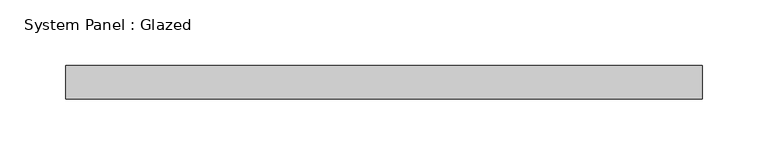
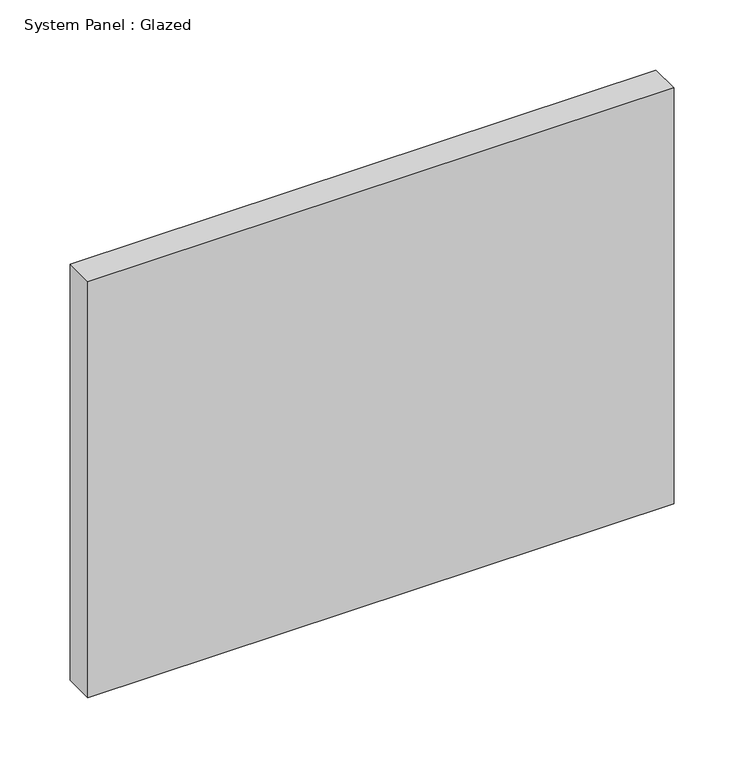
"""IFC4 building model written with IfcOpenShell, lengths in millimetres: plate geometry, System Panel : Glazed."""

from ifc_helpers import new_model, si_unit, origin, origin_with_axes, place, context, project, spatial, polyline, outline, extrude, source, transform, mapped, element, save


def system_panel_glazed_80b64450(model_context):
    return source(origin(), model_context, "Body", "SweptSolid", [
        extrude(outline(polyline([(241.3, -44.45), (-241.3, -44.45), (-241.3, -19.05), (241.3, -19.05), (241.3, -44.45)])), origin_with_axes(), (0.0, 0.0, 1.0), 361.95),
    ])


if __name__ == "__main__":
    model = new_model("IFC4")
    model_context = context("Model", 3, world=origin())
    ifc_project = project(units=[si_unit("LENGTHUNIT", "METRE", prefix="MILLI")], contexts=[model_context])
    site = spatial("IfcSite", under=ifc_project)
    building = spatial("IfcBuilding", under=site)
    placement = place(None, origin())
    system_panel_glazed_shape = system_panel_glazed_80b64450(model_context)
    element("IfcPlate", 1, ObjectType="System Panel : Glazed", at=placement, inside=building, context=model_context, shape_type="MappedRepresentation", body=[
        mapped(system_panel_glazed_shape, transform((0.0, 0.0, 0.0), x_axis=(1.0, 0.0, 0.0), y_axis=(0.0, 1.0, 0.0), z_axis=(0.0, 0.0, 1.0))),
    ])
    save(model, "model.ifc")

# Revit data of these elements
# Type "System Panel : Glazed"
#   Construction Type Id = "GSP4R"
#   Analytic Construction = "1/8 in Pilkington single glazing"
#   Visual Light Transmittance = 0.9
#   Solar Heat Gain Coefficient = 0.86
#   Heat Transfer Coefficient (U) = 1.18115 BTU/(h·ft²·°F)
#   Define Thermal Properties by = 1
# Element 1 (IfcPlate, "System Panel : Glazed")
#   Materials on its faces: "Glass"
# Materials
#   "Glass": class "Glass", colour RGB 0 128 192, transparency 0.75, Description = "Soda Lime Glass", Cost = 0
